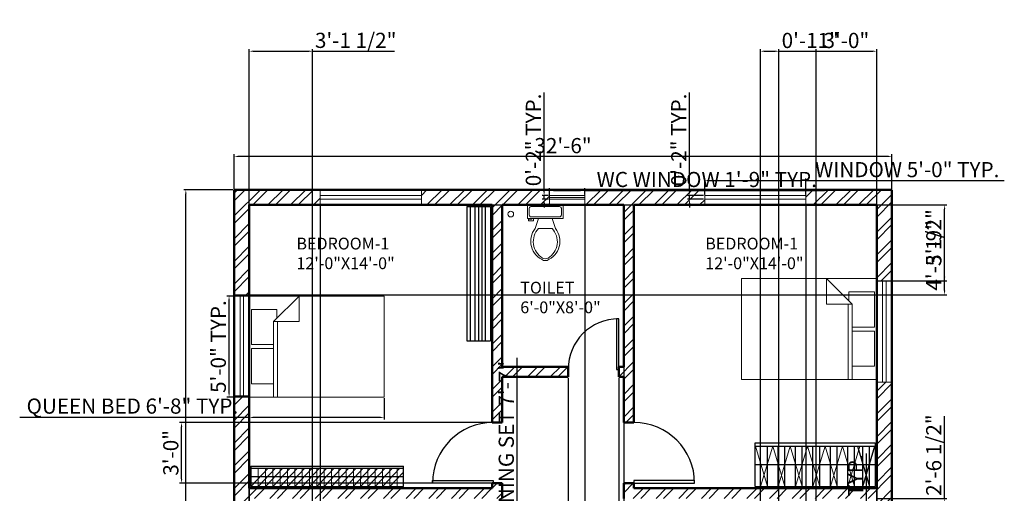
# Model space of a CAD drawing. Units: inches. Extents: x 1104 to 1745, y 678 to 1361.
# Tile 4 of 4: x 1104 to 1688, y 1080 to 1361. Entities that reach past the tile are written whole.
import ezdxf

# ---------------------------------------------------------------- set-up
doc = ezdxf.new("R2010")
doc.units = ezdxf.units.IN
doc.linetypes.add('ACAD_ISO02W100', pattern=[15, 12, -3])
for name, color, linetype, lineweight in [('A-ANNO-DIMS', 2, 'Continuous', 18), ('A-AREA-IDEN', 7, 'Continuous', 25), ('A-DOOR', 4, 'Continuous', 25), ('A-FLOR-CASE', 32, 'Continuous', 25), ('A-FLOR-CASE-PATT', 252, 'Continuous', 13), ('A-FLOR-FIXT', 8, 'Continuous', 18), ('A-FURN', 8, 'Continuous', 18), ('A-WALL', 7, 'Continuous', 50), ('A-WALL-PATT', 252, 'ACAD_ISO02W100', 13)]:
    doc.layers.add(name, color=color, linetype=linetype, lineweight=lineweight)
doc.layers.add('A-GLAZ', color=244, linetype='Continuous', lineweight=18, true_color=0x991b1e)
doc.styles.get("Standard").update_dxf_attribs({"font": 'arial.ttf'})
doc.dimstyles.new('ISO-25', dxfattribs={"dimtxt": 9, "dimasz": 2.5, "dimexe": 1.25, "dimexo": 0.625, "dimtad": 1, "dimlunit": 3, "dimtxsty": 'Standard', "dimcen": 2.5, "dimadec": 0, "dimazin": 0, "dimtfac": 1, "dimtmove": 0, "dimatfit": 3, "dimfxl": 1, "dimarcsym": 0})

# ---------------------------------------------------------------- blocks, each defined once
blk = doc.blocks.new('*U4')
for p, q in [((0, 0), (0, -6)), ((-40, 0), (-40, -6))]:
    blk.add_line(p, q)
blk.add_lwpolyline([(0, 0), (0, 40), (-1.75, 40), (-1.75, 0)], close=True)
blk.add_arc((0, 0), 40, 90, 180)
blk = doc.blocks.new('*U2')
for p, q in [((0, 0), (0, -6)), ((40, 0), (40, -6))]:
    blk.add_line(p, q)
blk.add_lwpolyline([(0, 0), (0, 40), (1.75, 40), (1.75, 0)], close=True)
blk.add_arc((0, 0), 40, 0, 90)
blk = doc.blocks.new('*U3')
for p, q in [((0, 0), (0, 6)), ((40, 0), (40, 6))]:
    blk.add_line(p, q)
blk.add_lwpolyline([(0, 0), (0, -40), (1.75, -40), (1.75, 0)], close=True)
blk.add_arc((0, 0), 40, 270, 0)
blk = doc.blocks.new('*D7')
at = {"layer": 'A-ANNO-DIMS', "color": 0, "lineweight": -2, "transparency": 16777216}
for p, q in [((1231.11, 1260.75), (1231.11, 1281.16)), ((1618.61, 1279.91), (1233.61, 1279.91)), ((1621.11, 1260.75), (1621.11, 1281.16))]:
    blk.add_line(p, q, dxfattribs=at)
at = {"layer": 'A-ANNO-DIMS', "color": 0, "transparency": 16777216}
for points in [[(1233.61, 1280.33), (1233.61, 1279.5), (1231.11, 1279.91)], [(1618.61, 1280.33), (1618.61, 1279.5), (1621.11, 1279.91)]]:
    blk.add_solid(points, dxfattribs=at)
at = {"layer": 'Defpoints', "color": 0, "transparency": 16777216}
for p in [(1231.11, 1279.91), (1231.11, 1260.13), (1621.11, 1260.13)]:
    blk.add_point(p, dxfattribs=at)
at = {"layer": 'A-ANNO-DIMS', "color": 0, "transparency": 16777216, "insert": (1426.11, 1285.14), "char_height": 9, "attachment_point": 5}
blk.add_mtext('32\'-6"', dxfattribs=at)
blk = doc.blocks.new('*D8')
at = {"layer": 'A-ANNO-DIMS', "color": 0, "lineweight": -2, "transparency": 16777216}
for p, q in [((1230.48, 1260.13), (1201.22, 1260.13)), ((1202.47, 722.45), (1202.47, 1257.63)), ((1230.48, 719.95), (1201.22, 719.95))]:
    blk.add_line(p, q, dxfattribs=at)
at = {"layer": 'A-ANNO-DIMS', "color": 0, "transparency": 16777216}
for points in [[(1202.05, 1257.63), (1202.88, 1257.63), (1202.47, 1260.13)], [(1202.05, 722.45), (1202.88, 722.45), (1202.47, 719.95)]]:
    blk.add_solid(points, dxfattribs=at)
at = {"layer": 'Defpoints', "color": 0, "transparency": 16777216}
for p in [(1202.47, 1260.13), (1231.11, 1260.13), (1231.11, 719.95)]:
    blk.add_point(p, dxfattribs=at)
at = {"layer": 'A-ANNO-DIMS', "color": 0, "transparency": 16777216, "insert": (1197.25, 990.04), "char_height": 9, "attachment_point": 5, "rotation": 90}
blk.add_mtext('45\'-0.18"', dxfattribs=at)
blk = doc.blocks.new('*U14')
for p, q in [((9.5, -6), (9.5, -2)), ((-10, -8.5), (-8, -8.5)), ((-10, -9.5), (-10, -8.5)), ((-7, -9.5), (-10, -9.5)), ((-8, -8.5), (-8, -8)), ((-7, -8), (-7, -9.5)), ((-4, -8), (-6, -14)), ((4, -8), (6, -14)), ((4, -14), (-4, -14))]:
    blk.add_line(p, q)
blk.add_lwpolyline([(10.5, -8), (10.5, 0), (-10.5, 0), (-10.5, -8)], close=True)
for points in [[(-9.5, -2), (-9.5, -6)], [(8.5, -1), (-8.5, -1)], [(-8.5, -7), (8.5, -7)]]:
    blk.add_lwpolyline(points)
for centre, radius, start, end in [((-8.62, -1.88), 0.884, 81.8699, 188.1301), ((8.62, -1.88), 0.884, 351.8699, 98.1301), ((-8.62, -6.12), 0.884, 171.8699, 278.1301), ((8.62, -6.12), 0.884, 261.8699, 8.1301), ((3.52, -21.58), 12.17, 141.46911, 247.97143), ((4.2, -21.82), 11.33, 136.36773, 238.94682), ((-3.52, -21.58), 12.17, 292.02843, 38.53071), ((-4.2, -21.82), 11.33, 301.05301, 43.63209), ((0, -27.88), 4, 245.73182, 294.26817), ((0, -29), 4, 254.86053, 285.13947)]:
    blk.add_arc(centre, radius, start, end)
blk = doc.blocks.new('Bed - Queen')
for p, q in [((0, -80.00003), (0, 0)), ((0, 0), (59.99999, 0)), ((59.99999, 0), (59.99999, -80.00003)), ((7.99999, -1.2), (28.79998, -1.2)), ((7.99999, -14.4), (7.99999, -1.2)), ((28.79998, -1.2), (28.79998, -14.4)), ((31.19999, -1.2), (51.99999, -1.2)), ((31.19999, -14.4), (31.19999, -1.2)), ((51.99999, -1.2), (51.99999, -16.4)), ((0, -14.4), (44.8, -14.4)), ((44.8, -16.8), (0, -16.8)), ((59.99999, -29.6), (44.8, -14.4)), ((44.8, -14.4), (44.8, -29.6)), ((51.99999, -16.4), (46.79936, -16.4)), ((44.8, -29.6), (59.99999, -29.6)), ((59.99999, -80.00003), (0, -80.00003))]:
    blk.add_line(p, q)
blk = doc.blocks.new('WIN-GLASS-60IN')
for p, q in [((0, 2), (60, 2)), ((0, 0), (60, 0))]:
    blk.add_line(p, q)
blk = doc.blocks.new('WIN-GLASS-21IN')
for p, q in [((0, 2), (21, 2)), ((0, 1), (21, 1)), ((0, 0), (21, 0))]:
    blk.add_line(p, q)
blk = doc.blocks.new('*D21')
at = {"layer": 'A-ANNO-DIMS', "color": 0, "lineweight": -2, "transparency": 16777216}
for p, q in [((1510.11, 1257.25), (1510.11, 1266.88)), ((1570.11, 1257.25), (1570.11, 1266.88)), ((1512.61, 1265.63), (1567.61, 1265.63)), ((1570.11, 1265.63), (1687.74, 1265.63))]:
    blk.add_line(p, q, dxfattribs=at)
at = {"layer": 'A-ANNO-DIMS', "color": 0, "transparency": 16777216}
for points in [[(1512.61, 1266.05), (1512.61, 1265.21), (1510.11, 1265.63)], [(1567.61, 1266.05), (1567.61, 1265.21), (1570.11, 1265.63)]]:
    blk.add_solid(points, dxfattribs=at)
at = {"layer": 'Defpoints', "color": 0, "transparency": 16777216}
for p in [(1570.11, 1265.63), (1510.11, 1256.63), (1570.11, 1256.63)]:
    blk.add_point(p, dxfattribs=at)
at = {"layer": 'A-ANNO-DIMS', "color": 0, "transparency": 16777216, "insert": (1630.18, 1270.91), "char_height": 9, "attachment_point": 5}
blk.add_mtext('WINDOW 5\'-0" TYP.', dxfattribs=at)
blk = doc.blocks.new('*D22')
at = {"layer": 'A-ANNO-DIMS', "color": 0, "lineweight": -2, "transparency": 16777216}
for p, q in [((1501.11, 1259.13), (1501.11, 1317.74)), ((1509.48, 1256.63), (1499.86, 1256.63)), ((1501.11, 1254.63), (1501.11, 1256.63)), ((1509.48, 1254.63), (1499.86, 1254.63)), ((1501.11, 1252.13), (1501.11, 1249.63))]:
    blk.add_line(p, q, dxfattribs=at)
at = {"layer": 'A-ANNO-DIMS', "color": 0, "transparency": 16777216}
for points in [[(1500.69, 1259.13), (1501.52, 1259.13), (1501.11, 1256.63)], [(1500.69, 1252.13), (1501.52, 1252.13), (1501.11, 1254.63)]]:
    blk.add_solid(points, dxfattribs=at)
at = {"layer": 'Defpoints', "color": 0, "transparency": 16777216}
for p in [(1501.11, 1256.63), (1510.11, 1256.63), (1510.11, 1254.63)]:
    blk.add_point(p, dxfattribs=at)
at = {"layer": 'A-ANNO-DIMS', "color": 0, "transparency": 16777216, "insert": (1495.89, 1289.68), "char_height": 9, "attachment_point": 5, "rotation": 90}
blk.add_mtext('0\'-2" TYP.', dxfattribs=at)
blk = doc.blocks.new('*D23')
at = {"layer": 'A-ANNO-DIMS', "color": 0, "lineweight": -2, "transparency": 16777216}
for p, q in [((1418.05, 1257.25), (1418.05, 1261.03)), ((1439.05, 1257.25), (1439.05, 1261.03)), ((1420.55, 1259.78), (1436.55, 1259.78)), ((1439.05, 1259.78), (1581.13, 1259.78))]:
    blk.add_line(p, q, dxfattribs=at)
at = {"layer": 'A-ANNO-DIMS', "color": 0, "transparency": 16777216}
for points in [[(1420.55, 1260.2), (1420.55, 1259.36), (1418.05, 1259.78)], [(1436.55, 1260.2), (1436.55, 1259.36), (1439.05, 1259.78)]]:
    blk.add_solid(points, dxfattribs=at)
at = {"layer": 'Defpoints', "color": 0, "transparency": 16777216}
for p in [(1418.05, 1256.63), (1439.05, 1259.78), (1439.05, 1256.63)]:
    blk.add_point(p, dxfattribs=at)
at = {"layer": 'A-ANNO-DIMS', "color": 0, "transparency": 16777216, "insert": (1511.34, 1265.06), "char_height": 9, "attachment_point": 5}
blk.add_mtext('WC WINDOW 1\'-9" TYP.', dxfattribs=at)
blk = doc.blocks.new('*D24')
at = {"layer": 'A-ANNO-DIMS', "color": 0, "lineweight": -2, "transparency": 16777216}
for p, q in [((1414.9, 1259.13), (1414.9, 1317.74)), ((1417.43, 1256.63), (1413.65, 1256.63)), ((1414.9, 1254.63), (1414.9, 1256.63)), ((1417.43, 1254.63), (1413.65, 1254.63)), ((1414.9, 1252.13), (1414.9, 1249.63))]:
    blk.add_line(p, q, dxfattribs=at)
at = {"layer": 'A-ANNO-DIMS', "color": 0, "transparency": 16777216}
for points in [[(1414.48, 1259.13), (1415.32, 1259.13), (1414.9, 1256.63)], [(1414.48, 1252.13), (1415.32, 1252.13), (1414.9, 1254.63)]]:
    blk.add_solid(points, dxfattribs=at)
at = {"layer": 'Defpoints', "color": 0, "transparency": 16777216}
for p in [(1414.9, 1256.63), (1418.05, 1256.63), (1418.05, 1254.63)]:
    blk.add_point(p, dxfattribs=at)
at = {"layer": 'A-ANNO-DIMS', "color": 0, "transparency": 16777216, "insert": (1409.68, 1289.68), "char_height": 9, "attachment_point": 5, "rotation": 90}
blk.add_mtext('0\'-2" TYP.', dxfattribs=at)
blk = doc.blocks.new('*D25')
at = {"layer": 'A-ANNO-DIMS', "color": 0, "lineweight": -2, "transparency": 16777216}
for p, q in [((1240.11, 1136.5), (1240.11, 1123.88)), ((1320.11, 1136.5), (1320.11, 1123.88)), ((1240.11, 1125.13), (1103.97, 1125.13)), ((1317.61, 1125.13), (1242.61, 1125.13))]:
    blk.add_line(p, q, dxfattribs=at)
at = {"layer": 'A-ANNO-DIMS', "color": 0, "transparency": 16777216}
for points in [[(1242.61, 1125.55), (1242.61, 1124.71), (1240.11, 1125.13)], [(1317.61, 1125.55), (1317.61, 1124.71), (1320.11, 1125.13)]]:
    blk.add_solid(points, dxfattribs=at)
at = {"layer": 'Defpoints', "color": 0, "transparency": 16777216}
for p in [(1240.11, 1137.13), (1320.11, 1137.13), (1240.11, 1125.13)]:
    blk.add_point(p, dxfattribs=at)
at = {"layer": 'A-ANNO-DIMS', "color": 0, "transparency": 16777216, "insert": (1170.79, 1130.68), "char_height": 9, "attachment_point": 5}
blk.add_mtext('QUEEN BED 6\'-8" TYP.', dxfattribs=at)
blk = doc.blocks.new('*D26')
at = {"layer": 'A-ANNO-DIMS', "color": 0, "lineweight": -2, "transparency": 16777216}
for p, q in [((1239.48, 1197.13), (1226.86, 1197.13)), ((1228.11, 1139.63), (1228.11, 1194.63)), ((1239.48, 1137.13), (1226.86, 1137.13))]:
    blk.add_line(p, q, dxfattribs=at)
at = {"layer": 'A-ANNO-DIMS', "color": 0, "transparency": 16777216}
for points in [[(1227.69, 1194.63), (1228.52, 1194.63), (1228.11, 1197.13)], [(1227.69, 1139.63), (1228.52, 1139.63), (1228.11, 1137.13)]]:
    blk.add_solid(points, dxfattribs=at)
at = {"layer": 'Defpoints', "color": 0, "transparency": 16777216}
for p in [(1228.11, 1197.13), (1240.11, 1197.13), (1240.11, 1137.13)]:
    blk.add_point(p, dxfattribs=at)
at = {"layer": 'A-ANNO-DIMS', "color": 0, "transparency": 16777216, "insert": (1222.89, 1167.13), "char_height": 9, "attachment_point": 5, "rotation": 90}
blk.add_mtext('5\'-0" TYP.', dxfattribs=at)
blk = doc.blocks.new('*D28')
at = {"layer": 'A-ANNO-DIMS', "color": 0, "lineweight": -2, "transparency": 16777216}
for p, q in [((1605.95, 1045.19), (1605.95, 1103.8)), ((1604.52, 1045.19), (1607.2, 1045.19)), ((1605.95, 1039.75), (1605.95, 1042.69)), ((1604.52, 1037.25), (1607.2, 1037.25))]:
    blk.add_line(p, q, dxfattribs=at)
at = {"layer": 'A-ANNO-DIMS', "color": 0, "transparency": 16777216}
for points in [[(1605.53, 1042.69), (1606.37, 1042.69), (1605.95, 1045.19)], [(1605.53, 1039.75), (1606.37, 1039.75), (1605.95, 1037.25)]]:
    blk.add_solid(points, dxfattribs=at)
at = {"layer": 'Defpoints', "color": 0, "transparency": 16777216}
for p in [(1603.9, 1045.19), (1605.95, 1045.19), (1603.9, 1037.25)]:
    blk.add_point(p, dxfattribs=at)
at = {"layer": 'A-ANNO-DIMS', "color": 0, "transparency": 16777216, "insert": (1600.73, 1075.75), "char_height": 9, "attachment_point": 5, "rotation": 90}
blk.add_mtext('0\'-8" TYP.', dxfattribs=at)
blk = doc.blocks.new('*D31')
at = {"layer": 'A-ANNO-DIMS', "color": 0, "lineweight": -2, "transparency": 16777216}
for p, q in [((1398.91, 1057.87), (1398.91, 1160.54)), ((1411.93, 1057.87), (1397.66, 1057.87)), ((1398.91, 969.37), (1398.91, 1055.37)), ((1411.93, 966.87), (1397.66, 966.87))]:
    blk.add_line(p, q, dxfattribs=at)
at = {"layer": 'A-ANNO-DIMS', "color": 0, "transparency": 16777216}
for points in [[(1398.49, 1055.37), (1399.32, 1055.37), (1398.91, 1057.87)], [(1398.49, 969.37), (1399.32, 969.37), (1398.91, 966.87)]]:
    blk.add_solid(points, dxfattribs=at)
at = {"layer": 'Defpoints', "color": 0, "transparency": 16777216}
for p in [(1398.91, 1057.87), (1412.56, 1057.87), (1412.56, 966.87)]:
    blk.add_point(p, dxfattribs=at)
at = {"layer": 'A-ANNO-DIMS', "color": 0, "transparency": 16777216, "insert": (1393.63, 1110.45), "char_height": 9, "attachment_point": 5, "rotation": 90}
blk.add_mtext('DINING SET 7\'-7"', dxfattribs=at)
blk = doc.blocks.new('*D38')
at = {"layer": 'A-ANNO-DIMS', "color": 0, "lineweight": -2, "transparency": 16777216}
for p, q in [((1389.48, 1122.13), (1198.71, 1122.13)), ((1199.96, 1088.63), (1199.96, 1119.63)), ((1389.48, 1086.13), (1198.71, 1086.13))]:
    blk.add_line(p, q, dxfattribs=at)
at = {"layer": 'A-ANNO-DIMS', "color": 0, "transparency": 16777216}
for points in [[(1199.54, 1119.63), (1200.37, 1119.63), (1199.96, 1122.13)], [(1199.54, 1088.63), (1200.37, 1088.63), (1199.96, 1086.13)]]:
    blk.add_solid(points, dxfattribs=at)
at = {"layer": 'Defpoints', "color": 0, "transparency": 16777216}
for p in [(1199.96, 1122.13), (1390.11, 1122.13), (1390.11, 1086.13)]:
    blk.add_point(p, dxfattribs=at)
at = {"layer": 'A-ANNO-DIMS', "color": 0, "transparency": 16777216, "insert": (1194.73, 1104.13), "char_height": 9, "attachment_point": 5, "rotation": 90}
blk.add_mtext('3\'-0"', dxfattribs=at)
blk = doc.blocks.new('*D39')
at = {"layer": 'A-ANNO-DIMS', "color": 0, "lineweight": -2, "transparency": 16777216}
for p, q in [((1429.11, 1148.5), (1429.11, 684.69)), ((1459.11, 1148.5), (1459.11, 684.69)), ((1431.61, 685.94), (1456.61, 685.94))]:
    blk.add_line(p, q, dxfattribs=at)
at = {"layer": 'A-ANNO-DIMS', "color": 0, "transparency": 16777216}
for points in [[(1431.61, 686.36), (1431.61, 685.52), (1429.11, 685.94)], [(1456.61, 686.36), (1456.61, 685.52), (1459.11, 685.94)]]:
    blk.add_solid(points, dxfattribs=at)
at = {"layer": 'Defpoints', "color": 0, "transparency": 16777216}
for p in [(1429.11, 1149.13), (1459.11, 1149.13), (1459.11, 685.94)]:
    blk.add_point(p, dxfattribs=at)
at = {"layer": 'A-ANNO-DIMS', "color": 0, "transparency": 16777216, "insert": (1444.11, 691.16), "char_height": 9, "attachment_point": 5}
blk.add_mtext('2\'-6"', dxfattribs=at)
blk = doc.blocks.new('*D40')
at = {"layer": 'A-ANNO-DIMS', "color": 0, "lineweight": -2, "transparency": 16777216}
for p, q in [((1240.11, 1250.5), (1240.11, 684.69)), ((1282.11, 1250.5), (1282.11, 684.69)), ((1242.61, 685.94), (1279.61, 685.94))]:
    blk.add_line(p, q, dxfattribs=at)
at = {"layer": 'A-ANNO-DIMS', "color": 0, "transparency": 16777216}
for points in [[(1242.61, 686.36), (1242.61, 685.52), (1240.11, 685.94)], [(1279.61, 686.36), (1279.61, 685.52), (1282.11, 685.94)]]:
    blk.add_solid(points, dxfattribs=at)
at = {"layer": 'Defpoints', "color": 0, "transparency": 16777216}
for p in [(1240.11, 1251.13), (1282.11, 1251.13), (1282.11, 685.94)]:
    blk.add_point(p, dxfattribs=at)
at = {"layer": 'A-ANNO-DIMS', "color": 0, "transparency": 16777216, "insert": (1261.11, 691.16), "char_height": 9, "attachment_point": 5}
blk.add_mtext('3\'-6"', dxfattribs=at)
blk = doc.blocks.new('*D41')
at = {"layer": 'A-ANNO-DIMS', "color": 0, "lineweight": -2, "transparency": 16777216}
for p, q in [((1240.73, 1251.13), (1653.59, 1251.13)), ((1652.34, 1200.34), (1652.34, 1248.63)), ((1240.73, 1197.84), (1653.59, 1197.84))]:
    blk.add_line(p, q, dxfattribs=at)
at = {"layer": 'A-ANNO-DIMS', "color": 0, "transparency": 16777216}
for points in [[(1651.93, 1248.63), (1652.76, 1248.63), (1652.34, 1251.13)], [(1651.93, 1200.34), (1652.76, 1200.34), (1652.34, 1197.84)]]:
    blk.add_solid(points, dxfattribs=at)
at = {"layer": 'Defpoints', "color": 0, "transparency": 16777216}
for p in [(1240.11, 1251.13), (1652.34, 1251.13), (1240.11, 1197.84)]:
    blk.add_point(p, dxfattribs=at)
at = {"layer": 'A-ANNO-DIMS', "color": 0, "transparency": 16777216, "insert": (1647.06, 1224.48), "char_height": 9, "attachment_point": 5, "rotation": 90}
blk.add_mtext('4\'-5 1/2"', dxfattribs=at)
blk = doc.blocks.new('*D48')
at = {"layer": 'A-ANNO-DIMS', "color": 0, "lineweight": -2, "transparency": 16777216}
for p, q in [((1612.73, 1251.13), (1653.59, 1251.13)), ((1652.34, 1208.59), (1652.34, 1248.63)), ((1612.73, 1206.09), (1653.59, 1206.09))]:
    blk.add_line(p, q, dxfattribs=at)
at = {"layer": 'A-ANNO-DIMS', "color": 0, "transparency": 16777216}
for points in [[(1651.93, 1248.63), (1652.76, 1248.63), (1652.34, 1251.13)], [(1651.93, 1208.59), (1652.76, 1208.59), (1652.34, 1206.09)]]:
    blk.add_solid(points, dxfattribs=at)
at = {"layer": 'Defpoints', "color": 0, "transparency": 16777216}
for p in [(1612.11, 1251.13), (1652.34, 1251.13), (1612.11, 1206.09)]:
    blk.add_point(p, dxfattribs=at)
at = {"layer": 'A-ANNO-DIMS', "color": 0, "transparency": 16777216, "insert": (1647.12, 1228.61), "char_height": 9, "attachment_point": 5, "rotation": 90}
blk.add_mtext('3\'-9"', dxfattribs=at)
blk = doc.blocks.new('*D49')
at = {"layer": 'A-ANNO-DIMS', "color": 0, "lineweight": -2, "transparency": 16777216}
for p, q in [((1652.34, 1077.13), (1652.34, 1125.93)), ((1612.73, 1077.13), (1653.59, 1077.13)), ((1652.34, 1049.17), (1652.34, 1074.63)), ((1621.73, 1046.67), (1653.59, 1046.67))]:
    blk.add_line(p, q, dxfattribs=at)
at = {"layer": 'A-ANNO-DIMS', "color": 0, "transparency": 16777216}
for points in [[(1651.93, 1074.63), (1652.76, 1074.63), (1652.34, 1077.13)], [(1651.93, 1049.17), (1652.76, 1049.17), (1652.34, 1046.67)]]:
    blk.add_solid(points, dxfattribs=at)
at = {"layer": 'Defpoints', "color": 0, "transparency": 16777216}
for p in [(1612.11, 1077.13), (1652.34, 1077.13), (1621.11, 1046.67)]:
    blk.add_point(p, dxfattribs=at)
at = {"layer": 'A-ANNO-DIMS', "color": 0, "transparency": 16777216, "insert": (1647.06, 1102.78), "char_height": 9, "attachment_point": 5, "rotation": 90}
blk.add_mtext('2\'-6 1/2"', dxfattribs=at)
blk = doc.blocks.new('*D53')
at = {"layer": 'A-ANNO-DIMS', "color": 0, "lineweight": -2, "transparency": 16777216}
for p, q in [((1576.11, 741.75), (1576.11, 1343.53)), ((1612.11, 741.75), (1612.11, 1343.53)), ((1578.61, 1342.28), (1609.61, 1342.28))]:
    blk.add_line(p, q, dxfattribs=at)
at = {"layer": 'A-ANNO-DIMS', "color": 0, "transparency": 16777216}
for points in [[(1578.61, 1342.7), (1578.61, 1341.86), (1576.11, 1342.28)], [(1609.61, 1342.7), (1609.61, 1341.86), (1612.11, 1342.28)]]:
    blk.add_solid(points, dxfattribs=at)
at = {"layer": 'Defpoints', "color": 0, "transparency": 16777216}
for p in [(1612.11, 1342.28), (1576.11, 741.13), (1612.11, 741.13)]:
    blk.add_point(p, dxfattribs=at)
at = {"layer": 'A-ANNO-DIMS', "color": 0, "transparency": 16777216, "insert": (1594.11, 1347.5), "char_height": 9, "attachment_point": 5}
blk.add_mtext('3\'-0"', dxfattribs=at)
blk = doc.blocks.new('*D55')
at = {"layer": 'A-ANNO-DIMS', "color": 0, "lineweight": -2, "transparency": 16777216}
for p, q in [((1543.11, 819.75), (1543.11, 1343.53)), ((1554.11, 819.75), (1554.11, 1343.53)), ((1545.61, 1342.28), (1551.61, 1342.28)), ((1554.11, 1342.28), (1588.77, 1342.28))]:
    blk.add_line(p, q, dxfattribs=at)
at = {"layer": 'A-ANNO-DIMS', "color": 0, "transparency": 16777216}
for points in [[(1545.61, 1342.7), (1545.61, 1341.86), (1543.11, 1342.28)], [(1551.61, 1342.7), (1551.61, 1341.86), (1554.11, 1342.28)]]:
    blk.add_solid(points, dxfattribs=at)
at = {"layer": 'Defpoints', "color": 0, "transparency": 16777216}
for p in [(1554.11, 1342.28), (1543.11, 819.13), (1554.11, 819.13)]:
    blk.add_point(p, dxfattribs=at)
at = {"layer": 'A-ANNO-DIMS', "color": 0, "transparency": 16777216, "insert": (1572.69, 1347.5), "char_height": 9, "attachment_point": 5}
blk.add_mtext('0\'-11"', dxfattribs=at)
blk = doc.blocks.new('*D56')
at = {"layer": 'A-ANNO-DIMS', "color": 0, "lineweight": -2, "transparency": 16777216}
for p, q in [((1240.11, 918.55), (1240.11, 1343.53)), ((1277.61, 918.55), (1277.61, 1343.53)), ((1242.61, 1342.28), (1275.11, 1342.28)), ((1277.61, 1342.28), (1326.25, 1342.28))]:
    blk.add_line(p, q, dxfattribs=at)
at = {"layer": 'A-ANNO-DIMS', "color": 0, "transparency": 16777216}
for points in [[(1242.61, 1342.7), (1242.61, 1341.86), (1240.11, 1342.28)], [(1275.11, 1342.7), (1275.11, 1341.86), (1277.61, 1342.28)]]:
    blk.add_solid(points, dxfattribs=at)
at = {"layer": 'Defpoints', "color": 0, "transparency": 16777216}
for p in [(1277.61, 1342.28), (1240.11, 917.92), (1277.61, 917.92)]:
    blk.add_point(p, dxfattribs=at)
at = {"layer": 'A-ANNO-DIMS', "color": 0, "transparency": 16777216, "insert": (1303.18, 1347.56), "char_height": 9, "attachment_point": 5}
blk.add_mtext('3\'-1 1/2"', dxfattribs=at)
blk = doc.blocks.new('*D57')
at = {"layer": 'A-ANNO-DIMS', "color": 0, "lineweight": -2, "transparency": 16777216}
for p, q in [((1439.05, 1250.5), (1439.05, 684.69)), ((1462.11, 1250.5), (1462.11, 684.69)), ((1441.55, 685.94), (1459.61, 685.94)), ((1462.11, 685.94), (1495.93, 685.94))]:
    blk.add_line(p, q, dxfattribs=at)
at = {"layer": 'A-ANNO-DIMS', "color": 0, "transparency": 16777216}
for points in [[(1441.55, 686.36), (1441.55, 685.52), (1439.05, 685.94)], [(1459.61, 686.36), (1459.61, 685.52), (1462.11, 685.94)]]:
    blk.add_solid(points, dxfattribs=at)
at = {"layer": 'Defpoints', "color": 0, "transparency": 16777216}
for p in [(1439.05, 1251.13), (1462.11, 1251.13), (1462.11, 685.94)]:
    blk.add_point(p, dxfattribs=at)
at = {"layer": 'A-ANNO-DIMS', "color": 0, "transparency": 16777216, "insert": (1480.27, 691.08), "char_height": 9, "attachment_point": 5}
blk.add_mtext('1\'-11"', dxfattribs=at)
blk = doc.blocks.new('*D58')
at = {"layer": 'A-ANNO-DIMS', "color": 0, "lineweight": -2, "transparency": 16777216}
for p, q in [((1570.11, 1250.5), (1570.11, 684.69)), ((1612.11, 1250.5), (1612.11, 684.69)), ((1572.61, 685.94), (1609.61, 685.94))]:
    blk.add_line(p, q, dxfattribs=at)
at = {"layer": 'A-ANNO-DIMS', "color": 0, "transparency": 16777216}
for points in [[(1572.61, 686.36), (1572.61, 685.52), (1570.11, 685.94)], [(1609.61, 686.36), (1609.61, 685.52), (1612.11, 685.94)]]:
    blk.add_solid(points, dxfattribs=at)
at = {"layer": 'Defpoints', "color": 0, "transparency": 16777216}
for p in [(1570.11, 1251.13), (1612.11, 1251.13), (1612.11, 685.94)]:
    blk.add_point(p, dxfattribs=at)
at = {"layer": 'A-ANNO-DIMS', "color": 0, "transparency": 16777216, "insert": (1591.11, 691.16), "char_height": 9, "attachment_point": 5}
blk.add_mtext('3\'-6"', dxfattribs=at)

msp = doc.modelspace()

# ---------------------------------------------------------------- hatches: boundary and pattern name
at = {"layer": 'A-FLOR-CASE-PATT'}
h = msp.add_hatch(dxfattribs=at)
h.set_pattern_fill('ANSI31', color=256, scale=3.11982, angle=61.6341, style=0)
h.paths.add_polyline_path([(1542.651, 1084.129), (1603.653, 1084.129), (1596.452, 1108.129), (1540.106, 1108.129), (1540.106, 1092.611)])
h = msp.add_hatch(dxfattribs=at)
h.set_pattern_fill('ANSI31', color=256, scale=3.12023, angle=28.3911, style=0)
h.paths.add_polyline_path([(1540.106, 1084.129), (1599.582, 1084.129), (1606.78, 1108.129), (1545.799, 1108.129), (1540.106, 1089.148)])
h = msp.add_hatch(dxfattribs=at)
h.set_pattern_fill('ANSI31', color=256, scale=0.998215, angle=1.98834, style=0)
h.paths.add_polyline_path([(1241.106, 1084.129), (1325.421, 1084.129), (1331.486, 1090.641), (1331.486, 1095.129), (1249.391, 1095.129), (1241.106, 1086.235)])
h = msp.add_hatch(dxfattribs=at)
h.set_pattern_fill('ANSI31', color=256, scale=1.365144, angle=44.92187, style=0)
h.paths.add_polyline_path([(1243.488, 1084.129), (1329.746, 1084.129), (1329.746, 1095.129), (1243.488, 1095.129)])
at = {"layer": 'A-WALL-PATT'}
h = msp.add_hatch(dxfattribs=at)
h.set_pattern_fill('ANSI32', color=256)
h.paths.add_polyline_path([(1277.606, 917.921), (1240.106, 917.921), (1240.106, 980.462), (1231.106, 980.462), (1231.106, 719.949), (1240.106, 719.949), (1240.106, 908.921), (1277.606, 908.921)])
h.paths.add_polyline_path([(1384.106, 917.921), (1337.606, 917.921), (1337.606, 908.921), (1375.106, 908.921), (1375.106, 836.921), (1387.106, 836.921), (1387.106, 844.121), (1387.106, 845.921), (1384.106, 845.921)])
h.paths.add_polyline_path([(1486.106, 849.129), (1543.106, 849.129), (1543.106, 855.129), (1540.106, 855.129), (1540.106, 951.129), (1612.106, 951.129), (1612.106, 941.864), (1621.106, 941.864), (1621.106, 986.665), (1612.106, 986.665), (1612.106, 957.129), (1486.106, 957.129), (1486.106, 1017.129), (1480.106, 1017.129), (1480.106, 951.129), (1534.106, 951.129), (1534.106, 855.129), (1480.106, 855.129), (1480.106, 845.921), (1476.166, 845.921), (1476.166, 836.921), (1480.106, 836.921), (1480.106, 833.921), (1486.106, 833.921)])
h.paths.add_polyline_path([(1441.89, 845.921), (1435.106, 845.921), (1435.106, 836.921), (1441.89, 836.921)])
h.paths.add_polyline_path([(1240.106, 1137.841), (1231.106, 1137.841), (1231.106, 1040.462), (1240.106, 1040.462), (1240.106, 1077.129), (1390.106, 1077.129), (1390.106, 1086.129), (1384.106, 1086.129), (1384.106, 1083.129), (1240.106, 1083.129)])
h.paths.add_polyline_path([(1621.106, 1146.091), (1612.106, 1146.091), (1612.106, 1083.129), (1468.106, 1083.129), (1468.106, 1086.129), (1462.106, 1086.129), (1462.106, 1077.129), (1480.106, 1077.129), (1612.106, 1077.129), (1612.106, 1046.665), (1621.106, 1046.665)])
h.paths.add_polyline_path([(1240.106, 1251.129), (1282.106, 1251.129), (1282.106, 1260.129), (1231.106, 1260.129), (1231.106, 1197.841), (1240.106, 1197.841)])
h.paths.add_polyline_path([(1418.05, 1260.129), (1342.106, 1260.129), (1342.106, 1251.129), (1384.106, 1251.129), (1384.106, 1122.129), (1390.106, 1122.129), (1390.106, 1149.129), (1429.106, 1149.129), (1429.106, 1155.129), (1390.106, 1155.129), (1390.106, 1251.129), (1418.05, 1251.129)])
h.paths.add_polyline_path([(1510.106, 1260.129), (1439.05, 1260.129), (1439.05, 1251.129), (1462.106, 1251.129), (1462.106, 1155.129), (1459.106, 1155.129), (1459.106, 1153.629), (1459.106, 1149.129), (1462.106, 1149.129), (1462.106, 1122.129), (1468.106, 1122.129), (1468.106, 1251.129), (1510.106, 1251.129)])
h.paths.add_polyline_path([(1621.106, 1260.129), (1570.106, 1260.129), (1570.106, 1251.129), (1612.106, 1251.129), (1612.106, 1206.091), (1621.106, 1206.091)])
h.paths.add_polyline_path([(1621.106, 920.864), (1612.106, 920.864), (1612.106, 855.129), (1573.106, 855.129), (1573.106, 849.129), (1612.106, 849.129), (1612.106, 809.56), (1621.106, 809.56)])
h.paths.add_polyline_path([(1621.106, 749.56), (1612.106, 749.56), (1612.106, 741.129), (1486.106, 741.129), (1486.106, 797.921), (1480.106, 797.921), (1480.106, 732.129), (1621.106, 732.129)])

# ---------------------------------------------------------------- linework, layer by layer
at = {"layer": 'A-FLOR-CASE'}
for p, q in [((1369.106, 1250.129), (1383.106, 1250.129)), ((1369.106, 1250.129), (1369.106, 1170.547)), ((1371.106, 1250.129), (1371.106, 1170.547)), ((1374.106, 1170.547), (1374.106, 1250.129)), ((1376.106, 1170.547), (1376.106, 1250.129)), ((1378.106, 1170.547), (1378.106, 1250.129)), ((1380.106, 1170.547), (1380.106, 1250.129)), ((1383.106, 1250.129), (1383.106, 1170.547)), ((1369.106, 1170.547), (1383.106, 1170.547)), ((1540.106, 1084.129), (1540.106, 1110.129)), ((1540.106, 1110.129), (1611.106, 1110.129)), ((1611.106, 1110.129), (1611.106, 1084.129)), ((1540.106, 1108.129), (1611.106, 1108.129)), ((1543.247, 1084.129), (1543.247, 1108.129)), ((1547.307, 1084.129), (1547.307, 1108.129)), ((1553.585, 1084.129), (1553.585, 1108.129)), ((1557.645, 1084.129), (1557.645, 1108.129)), ((1563.923, 1084.129), (1563.923, 1108.129)), ((1567.983, 1084.129), (1567.983, 1108.129)), ((1574.261, 1084.129), (1574.261, 1108.129)), ((1578.321, 1084.129), (1578.321, 1108.129)), ((1584.599, 1084.129), (1584.599, 1108.129)), ((1588.659, 1084.129), (1588.659, 1108.129)), ((1594.937, 1084.129), (1594.937, 1108.129)), ((1598.997, 1084.129), (1598.997, 1108.129)), ((1600.639, 1108.129), (1607.84, 1084.129)), ((1603.779, 1084.129), (1603.779, 1108.129)), ((1603.779, 1084.129), (1610.977, 1108.129)), ((1607.84, 1084.129), (1607.84, 1108.129)), ((1241.106, 1096.129), (1331.486, 1096.129)), ((1241.106, 1096.129), (1241.106, 1084.129)), ((1241.106, 1095.129), (1331.486, 1095.129)), ((1331.486, 1084.129), (1331.486, 1096.129)), ((1540.106, 1097.129), (1611.106, 1097.129)), ((1241.106, 1090.129), (1331.486, 1090.129)), ((1241.106, 1084.129), (1331.486, 1084.129)), ((1540.106, 1084.129), (1611.106, 1084.129))]:
    msp.add_line(p, q, dxfattribs=at)
at = {"layer": 'A-FLOR-FIXT'}
msp.add_circle((1395.122, 1245.692), 1.709, dxfattribs=at)
at = {"layer": 'A-GLAZ'}
for points in [[(1282.106, 1260.129), (1342.106, 1260.129), (1342.106, 1251.129), (1282.106, 1251.129)], [(1418.05, 1260.129), (1439.05, 1260.129), (1439.05, 1251.129), (1418.05, 1251.129)], [(1510.106, 1260.129), (1570.106, 1260.129), (1570.106, 1251.129), (1510.106, 1251.129)], [(1621.106, 1206.091), (1621.106, 1146.091), (1612.106, 1146.091), (1612.106, 1206.091)], [(1240.106, 1197.841), (1240.106, 1137.841), (1231.106, 1137.841), (1231.106, 1197.841)]]:
    msp.add_lwpolyline(points, close=True, dxfattribs=at)
at = {"layer": 'A-WALL'}
for p, q in [((1231.106, 1260.129), (1231.106, 719.949)), ((1231.106, 1260.129), (1621.106, 1260.129)), ((1621.106, 1260.129), (1621.106, 732.129)), ((1240.106, 1251.129), (1240.106, 1083.129)), ((1240.106, 1251.129), (1384.106, 1251.129)), ((1384.106, 1251.129), (1384.106, 1122.129)), ((1390.106, 1251.129), (1390.106, 1155.129)), ((1390.106, 1251.129), (1462.106, 1251.129)), ((1462.106, 1251.129), (1462.106, 1155.129)), ((1468.106, 1251.129), (1468.106, 1122.129)), ((1468.106, 1251.129), (1612.106, 1251.129)), ((1612.106, 1251.129), (1612.106, 1083.129)), ((1390.106, 1155.129), (1429.106, 1155.129)), ((1429.106, 1155.129), (1429.106, 1149.129)), ((1459.106, 1155.129), (1459.106, 1149.129)), ((1459.106, 1155.129), (1462.106, 1155.129)), ((1390.106, 1149.129), (1429.106, 1149.129)), ((1390.106, 1149.129), (1390.106, 1122.129)), ((1459.106, 1149.129), (1462.106, 1149.129)), ((1462.106, 1149.129), (1462.106, 1122.129)), ((1384.106, 1122.129), (1390.106, 1122.129)), ((1468.106, 1122.129), (1462.106, 1122.129)), ((1384.106, 1086.129), (1390.106, 1086.129)), ((1384.106, 1086.129), (1384.106, 1083.129)), ((1390.106, 1086.129), (1390.106, 1077.129)), ((1468.106, 1086.129), (1462.106, 1086.129)), ((1462.106, 1086.129), (1462.106, 1077.129)), ((1468.106, 1086.129), (1468.106, 1083.129)), ((1240.106, 1083.129), (1384.106, 1083.129)), ((1468.106, 1083.129), (1612.106, 1083.129))]:
    msp.add_line(p, q, dxfattribs=at)

# ---------------------------------------------------------------- block references
at = {"layer": 'A-DOOR', "xscale": 0.7499999999999887, "yscale": 0.7499999999999887, "zscale": 0.7499999999999887}
msp.add_blockref('*U4', (1459.106, 1153.629), dxfattribs=at)
at = {"layer": 'A-DOOR', "xscale": 0.9000000000000049, "yscale": 0.9000000000000049, "zscale": 0.9000000000000049, "rotation": 90}
for name, p in [('*U2', (1384.706, 1086.129)), ('*U3', (1468.106, 1086.129))]:
    msp.add_blockref(name, p, dxfattribs=at)
at = {"layer": 'A-FLOR-FIXT'}
msp.add_blockref('*U14', (1415.606, 1251.129), dxfattribs=at)
at = {"layer": 'A-FURN', "xscale": -1, "rotation": 270}
msp.add_blockref('Bed - Queen', (1611.912, 1147.529), dxfattribs=at)
at = {"layer": 'A-FURN', "rotation": 90}
msp.add_blockref('Bed - Queen', (1240.106, 1137.129), dxfattribs=at)
at = {"layer": 'A-GLAZ'}
for name, p in [('WIN-GLASS-60IN', (1282.106, 1254.629)), ('WIN-GLASS-21IN', (1418.05, 1254.629)), ('WIN-GLASS-60IN', (1510.106, 1254.629))]:
    msp.add_blockref(name, p, dxfattribs=at)
for p, rotation in [((1615.607, 1206.092), 269.9999999999992), ((1234.607, 1197.841), 270)]:
    msp.add_blockref('WIN-GLASS-60IN', p, dxfattribs=dict(at, rotation=rotation))

# ---------------------------------------------------------------- texts
at = {"layer": 'A-AREA-IDEN', "char_height": 7, "attachment_point": 1}
for s, width, insert in [('BEDROOM-1\\P12\'-0"X14\'-0"', 66.12074, (1268.038, 1231.711)), ('BEDROOM-1\\P12\'-0"X14\'-0"', 66.12074, (1510.426, 1231.711)), ('TOILET\\P6\'-0"X8\'-0"', 43.94389, (1400.762, 1205.567))]:
    msp.add_mtext_dynamic_manual_height_columns(s, width=width, gutter_width=12.5, heights=[0], dxfattribs=dict(at, insert=insert))

# ---------------------------------------------------------------- dimensions: what is measured, and where the dimension line sits
at = {"layer": 'A-ANNO-DIMS'}
for base, p1, p2, override, picture, middle in [((1277.606, 1342.279), (1240.106, 917.921), (1277.606, 917.921), {"dimdec": 1, "dimlfac": 1, "dimrnd": 0, "dimzin": 1, "dimdsep": 46, "dimlunit": 4, "dimfrac": 2}, '*D56', (1303.176, 1347.56)), ((1554.106, 1342.279), (1543.106, 819.129), (1554.106, 819.129), {"dimdec": 1, "dimlfac": 1, "dimrnd": 0, "dimzin": 1, "dimdsep": 46, "dimlunit": 4, "dimfrac": 2}, '*D55', (1572.69, 1347.499)), ((1612.106, 1342.279), (1576.106, 741.129), (1612.106, 741.129), {"dimdec": 1, "dimlfac": 1, "dimrnd": 0, "dimzin": 1, "dimdsep": 46, "dimlunit": 4, "dimfrac": 2}, '*D53', (1594.106, 1347.502)), ((1231.106, 1279.915), (1621.106, 1260.129), (1231.106, 1260.129), {"dimclrd": 0, "dimclre": 0, "dimclrt": 0}, '*D7', (1426.106, 1285.138)), ((1282.106, 685.941), (1240.106, 1251.129), (1282.106, 1251.129), {"dimdec": 1, "dimlfac": 1, "dimrnd": 0, "dimzin": 1, "dimdsep": 46, "dimlunit": 4, "dimfrac": 2}, '*D40', (1261.106, 691.164)), ((1462.106, 685.941), (1439.05, 1251.129), (1462.106, 1251.129), {"dimdec": 1, "dimlfac": 1, "dimrnd": 0, "dimzin": 1, "dimdsep": 46, "dimlunit": 4, "dimfrac": 2}, '*D57', (1480.266, 691.084)), ((1612.106, 685.941), (1570.106, 1251.129), (1612.106, 1251.129), {"dimdec": 1, "dimlfac": 1, "dimrnd": 0, "dimzin": 1, "dimdsep": 46, "dimlunit": 4, "dimfrac": 2}, '*D58', (1591.106, 691.164)), ((1459.106, 685.941), (1429.106, 1149.129), (1459.106, 1149.129), {"dimdec": 1, "dimlfac": 1, "dimrnd": 0, "dimzin": 1, "dimdsep": 46, "dimlunit": 4, "dimfrac": 2}, '*D39', (1444.106, 691.161))]:
    dim = msp.add_linear_dim(base=base, p1=p1, p2=p2, dimstyle='ISO-25', override=override, dxfattribs=at)
    dim.commit()
    dim.dimension.update_dxf_attribs({"geometry": picture, "text_midpoint": middle})
for base, p1, p2, angle, text, picture, middle in [((1414.9, 1256.629), (1418.05, 1254.629), (1418.05, 1256.629), 90, '<> TYP.', '*D24', (1409.68, 1289.683)), ((1501.106, 1256.629), (1510.106, 1254.629), (1510.106, 1256.629), 90, '<> TYP.', '*D22', (1495.886, 1289.683)), ((1228.106, 1197.129), (1240.106, 1137.129), (1240.106, 1197.129), 90, '<> TYP.', '*D26', (1222.886, 1167.129)), ((1240.106, 1125.129), (1320.107, 1137.129), (1240.106, 1137.129), 180, 'QUEEN BED <> TYP.', '*D25', (1170.786, 1130.683)), ((1398.906, 1057.865), (1412.556, 966.865), (1412.556, 1057.865), 90, 'DINING SET <>', '*D31', (1393.627, 1110.45)), ((1605.95, 1045.194), (1603.897, 1037.25), (1603.897, 1045.194), 90, '<> TYP.', '*D28', (1600.73, 1075.749))]:
    dim = msp.add_linear_dim(base=base, p1=p1, p2=p2, angle=angle, text=text, dimstyle='ISO-25', override={"dimdec": 1, "dimlfac": 1, "dimrnd": 0, "dimzin": 1, "dimdsep": 46, "dimlunit": 4, "dimfrac": 2}, dxfattribs=at)
    dim.commit()
    dim.dimension.update_dxf_attribs({"geometry": picture, "text_midpoint": middle})
for base, p1, p2, text, picture, middle in [((1439.05, 1259.779), (1418.05, 1256.629), (1439.05, 1256.629), 'WC WINDOW <> TYP.', '*D23', (1511.339, 1265.06)), ((1570.106, 1265.629), (1510.106, 1256.629), (1570.106, 1256.629), 'WINDOW <> TYP.', '*D21', (1630.175, 1270.91))]:
    dim = msp.add_linear_dim(base=base, p1=p1, p2=p2, text=text, dimstyle='ISO-25', override={"dimdec": 1, "dimlfac": 1, "dimrnd": 0, "dimzin": 1, "dimdsep": 46, "dimlunit": 4, "dimfrac": 2}, dxfattribs=at)
    dim.commit()
    dim.dimension.update_dxf_attribs({"geometry": picture, "text_midpoint": middle})
for base, p1, p2, override, picture, middle in [((1202.467, 1260.129), (1231.106, 719.949), (1231.106, 1260.129), {"dimclrd": 0, "dimclre": 0, "dimclrt": 0}, '*D8', (1197.247, 990.039)), ((1652.342, 1251.129), (1240.106, 1197.841), (1240.106, 1251.129), {"dimdec": 1, "dimlfac": 1, "dimrnd": 0, "dimzin": 1, "dimdsep": 46, "dimlunit": 4, "dimfrac": 2}, '*D41', (1647.064, 1224.485)), ((1652.342, 1251.129), (1612.106, 1206.091), (1612.106, 1251.129), {"dimdec": 1, "dimlfac": 1, "dimrnd": 0, "dimzin": 1, "dimdsep": 46, "dimlunit": 4, "dimfrac": 2}, '*D48', (1647.119, 1228.61)), ((1199.956, 1122.129), (1390.106, 1086.129), (1390.106, 1122.129), {"dimdec": 1, "dimlfac": 1, "dimrnd": 0, "dimzin": 1, "dimdsep": 46, "dimlunit": 4, "dimfrac": 2}, '*D38', (1194.733, 1104.129)), ((1652.342, 1077.129), (1621.106, 1046.665), (1612.106, 1077.129), {"dimdec": 1, "dimlfac": 1, "dimrnd": 0, "dimzin": 1, "dimdsep": 46, "dimlunit": 4, "dimfrac": 2}, '*D49', (1647.064, 1102.778))]:
    dim = msp.add_linear_dim(base=base, p1=p1, p2=p2, angle=90, dimstyle='ISO-25', override=override, dxfattribs=at)
    dim.commit()
    dim.dimension.update_dxf_attribs({"geometry": picture, "text_midpoint": middle})

doc.saveas('drawing.dxf')
